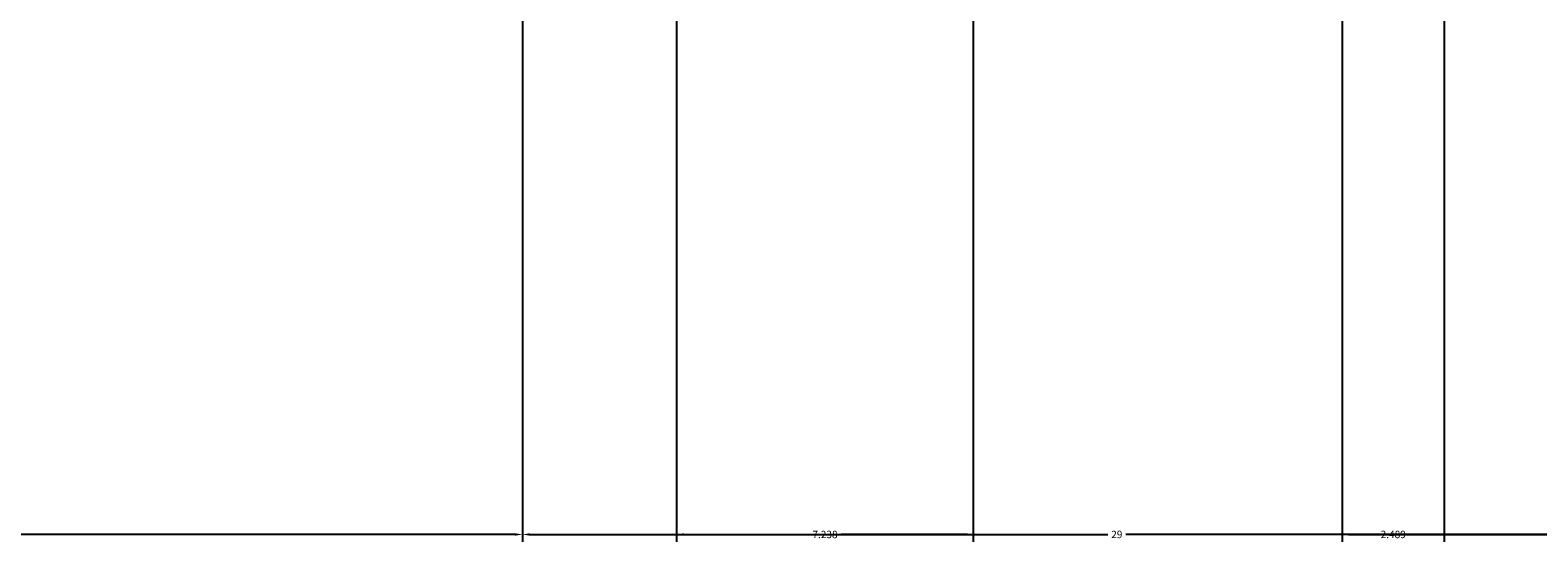
# Model space of a CAD drawing. Units: inches. Extents: x 2812 to 3051, y 1398 to 1659.
# Tile 19 of 65: x 2929 to 2966, y 1398 to 1410. Entities that reach past the tile are written whole.
import ezdxf

# ---------------------------------------------------------------- set-up
doc = ezdxf.new("R2010")
doc.units = ezdxf.units.IN
doc.layers.add('A-ANNO-DIMS', color=2, linetype='Continuous', lineweight=18)
doc.styles.get("Standard").update_dxf_attribs({"font": 'arial.ttf'})
doc.dimstyles.get("Standard").update_dxf_attribs({"dimtxt": 0.18, "dimasz": 0.18, "dimexe": 0.18, "dimexo": 0.0625, "dimgap": 0.09, "dimtad": 0, "dimtih": 1, "dimtoh": 1, "dimdec": 4, "dimzin": 0, "dimdsep": 46, "dimtxsty": 'Standard', "dimcen": 0.09, "dimadec": 0, "dimazin": 0, "dimtfac": 1, "dimtdec": 4, "dimtofl": 0, "dimtmove": 0, "dimatfit": 3, "dimfxl": 1, "dimtolj": 1, "dimtzin": 0, "dimarcsym": 0})

# ---------------------------------------------------------------- blocks, each defined once
blk = doc.blocks.new('*D30')
at = {"layer": 'A-ANNO-DIMS', "color": 0, "lineweight": -2, "transparency": 16777216}
for p, q in [((2945.147, 1598.692), (2945.147, 1397.505)), ((2952.385, 1559.757), (2952.385, 1397.505)), ((2945.327, 1397.685), (2948.373, 1397.685)), ((2952.205, 1397.685), (2949.159, 1397.685))]:
    blk.add_line(p, q, dxfattribs=at)
at = {"layer": 'A-ANNO-DIMS', "color": 0, "transparency": 16777216}
for points in [[(2945.327, 1397.715), (2945.327, 1397.655), (2945.147, 1397.685)], [(2952.205, 1397.715), (2952.205, 1397.655), (2952.385, 1397.685)]]:
    blk.add_solid(points, dxfattribs=at)
at = {"layer": 'Defpoints', "color": 0, "transparency": 16777216}
for p in [(2945.147, 1598.754), (2952.385, 1559.82), (2952.385, 1397.685)]:
    blk.add_point(p, dxfattribs=at)
at = {"layer": 'A-ANNO-DIMS', "color": 0, "transparency": 16777216, "insert": (2948.766, 1397.685), "char_height": 0.18, "attachment_point": 5}
blk.add_mtext('\\A1;7.238', dxfattribs=at)
blk = doc.blocks.new('*D31')
at = {"layer": 'A-ANNO-DIMS', "color": 0, "lineweight": -2, "transparency": 16777216}
for p, q in [((2972.272, 1594.192), (2972.272, 1397.505)), ((2961.385, 1559.757), (2961.385, 1397.505)), ((2961.565, 1397.685), (2966.373, 1397.685)), ((2972.092, 1397.685), (2967.283, 1397.685))]:
    blk.add_line(p, q, dxfattribs=at)
at = {"layer": 'A-ANNO-DIMS', "color": 0, "transparency": 16777216}
for points in [[(2961.565, 1397.715), (2961.565, 1397.655), (2961.385, 1397.685)], [(2972.092, 1397.715), (2972.092, 1397.655), (2972.272, 1397.685)]]:
    blk.add_solid(points, dxfattribs=at)
at = {"layer": 'Defpoints', "color": 0, "transparency": 16777216}
for p in [(2972.272, 1594.254), (2961.385, 1559.82), (2972.272, 1397.685)]:
    blk.add_point(p, dxfattribs=at)
at = {"layer": 'A-ANNO-DIMS', "color": 0, "transparency": 16777216, "insert": (2966.828, 1397.685), "char_height": 0.18, "attachment_point": 5}
blk.add_mtext('\\A1;10.887', dxfattribs=at)
blk = doc.blocks.new('*D45')
at = {"layer": 'A-ANNO-DIMS', "color": 0, "lineweight": -2, "transparency": 16777216}
for p, q in [((2896.385, 1487.973), (2896.385, 1397.505)), ((2941.385, 1487.973), (2941.385, 1397.505)), ((2896.565, 1397.685), (2918.662, 1397.685)), ((2941.205, 1397.685), (2919.108, 1397.685))]:
    blk.add_line(p, q, dxfattribs=at)
at = {"layer": 'A-ANNO-DIMS', "color": 0, "transparency": 16777216}
for points in [[(2896.565, 1397.715), (2896.565, 1397.655), (2896.385, 1397.685)], [(2941.205, 1397.715), (2941.205, 1397.655), (2941.385, 1397.685)]]:
    blk.add_solid(points, dxfattribs=at)
at = {"layer": 'Defpoints', "color": 0, "transparency": 16777216}
for p in [(2896.385, 1488.035), (2941.385, 1488.035), (2941.385, 1397.685)]:
    blk.add_point(p, dxfattribs=at)
at = {"layer": 'A-ANNO-DIMS', "color": 0, "transparency": 16777216, "insert": (2918.885, 1397.685), "char_height": 0.18, "attachment_point": 5}
blk.add_mtext('\\A1;45', dxfattribs=at)
blk = doc.blocks.new('*D46')
at = {"layer": 'A-ANNO-DIMS', "color": 0, "lineweight": -2, "transparency": 16777216}
for p, q in [((2941.385, 1487.973), (2941.385, 1397.505)), ((2970.385, 1487.973), (2970.385, 1397.505)), ((2941.565, 1397.685), (2955.664, 1397.685)), ((2970.205, 1397.685), (2956.106, 1397.685))]:
    blk.add_line(p, q, dxfattribs=at)
at = {"layer": 'A-ANNO-DIMS', "color": 0, "transparency": 16777216}
for points in [[(2941.565, 1397.715), (2941.565, 1397.655), (2941.385, 1397.685)], [(2970.205, 1397.715), (2970.205, 1397.655), (2970.385, 1397.685)]]:
    blk.add_solid(points, dxfattribs=at)
at = {"layer": 'Defpoints', "color": 0, "transparency": 16777216}
for p in [(2941.385, 1488.035), (2970.385, 1488.035), (2970.385, 1397.685)]:
    blk.add_point(p, dxfattribs=at)
at = {"layer": 'A-ANNO-DIMS', "color": 0, "transparency": 16777216, "insert": (2955.885, 1397.685), "char_height": 0.18, "attachment_point": 5}
blk.add_mtext('\\A1;29', dxfattribs=at)
blk = doc.blocks.new('*D70')
at = {"layer": 'A-ANNO-DIMS', "color": 0, "lineweight": -2, "transparency": 16777216}
for p, q in [((2961.385, 1450.411), (2961.385, 1397.505)), ((2963.874, 1450.411), (2963.874, 1397.505)), ((2961.565, 1397.685), (2962.234, 1397.685)), ((2963.694, 1397.685), (2963.025, 1397.685))]:
    blk.add_line(p, q, dxfattribs=at)
at = {"layer": 'A-ANNO-DIMS', "color": 0, "transparency": 16777216}
for points in [[(2961.565, 1397.715), (2961.565, 1397.655), (2961.385, 1397.685)], [(2963.694, 1397.715), (2963.694, 1397.655), (2963.874, 1397.685)]]:
    blk.add_solid(points, dxfattribs=at)
at = {"layer": 'Defpoints', "color": 0, "transparency": 16777216}
for p in [(2961.385, 1450.474), (2963.874, 1450.474), (2963.874, 1397.685)]:
    blk.add_point(p, dxfattribs=at)
at = {"layer": 'A-ANNO-DIMS', "color": 0, "transparency": 16777216, "insert": (2962.63, 1397.685), "char_height": 0.18, "attachment_point": 5}
blk.add_mtext('\\A1;2.489', dxfattribs=at)

msp = doc.modelspace()

# ---------------------------------------------------------------- dimensions: what is measured, and where the dimension line sits
at = {"layer": 'A-ANNO-DIMS'}
for base, p1, p2, override, picture, middle in [((2952.3849, 1397.6854), (2945.1467, 1598.7541), (2952.3849, 1559.82), {"dimdec": 3, "dimlfac": 1, "dimrnd": 0, "dimzin": 0, "dimdsep": 46, "dimlunit": 2}, '*D30', (2948.7658, 1397.6854)), ((2972.2716, 1397.6854), (2961.3849, 1559.82), (2972.2716, 1594.2541), {"dimdec": 3, "dimlfac": 1, "dimrnd": 0, "dimzin": 0, "dimdsep": 46, "dimlunit": 2}, '*D31', (2966.8282, 1397.6854)), ((2941.3849, 1397.6854), (2896.3849, 1488.0354), (2941.3849, 1488.0354), {"dimdec": 0, "dimlfac": 1, "dimrnd": 0, "dimzin": 0, "dimdsep": 46, "dimlunit": 2}, '*D45', (2918.8849, 1397.6854)), ((2970.3849, 1397.6854), (2941.3849, 1488.0354), (2970.3849, 1488.0354), {"dimdec": 0, "dimlfac": 1, "dimrnd": 0, "dimzin": 0, "dimdsep": 46, "dimlunit": 2}, '*D46', (2955.8849, 1397.6854)), ((2963.8741, 1397.6854), (2961.3849, 1450.4738), (2963.8741, 1450.4738), {"dimdec": 3, "dimlfac": 1, "dimrnd": 0, "dimzin": 0, "dimdsep": 46, "dimlunit": 2}, '*D70', (2962.6295, 1397.6854))]:
    dim = msp.add_linear_dim(base=base, p1=p1, p2=p2, dimstyle='Standard', override=override, dxfattribs=at)
    dim.commit()
    dim.dimension.update_dxf_attribs({"geometry": picture, "text_midpoint": middle})

doc.saveas('drawing.dxf')
